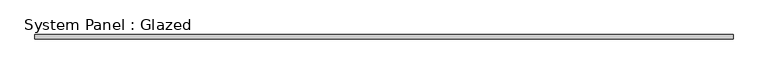
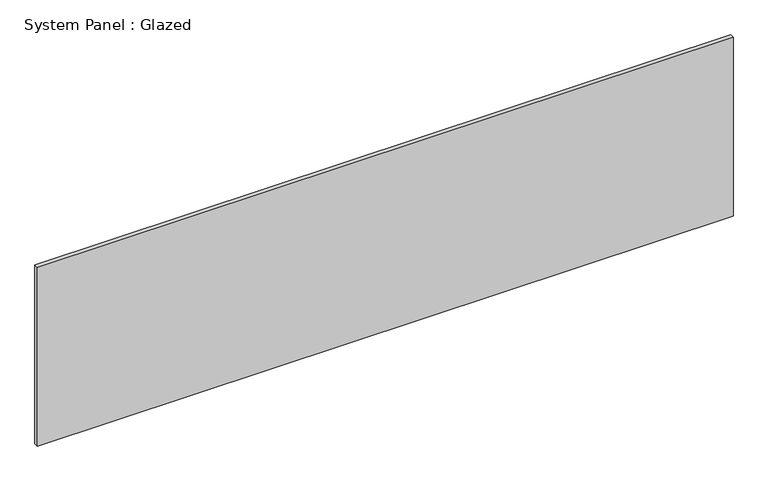
"""IFC4 building model written with IfcOpenShell, lengths in millimetres: plate geometry, System Panel : Glazed."""

from ifc_helpers import new_model, si_unit, origin, origin_with_axes, place, context, project, spatial, polyline, outline, extrude, source, transform, mapped, element, save


def system_panel_glazed_93b9a344(model_context):
    return source(origin(), model_context, "Body", "SweptSolid", [
        extrude(outline(polyline([(2009.775, 19.05), (-2009.775, 19.05), (-2009.775, 44.45), (2009.775, 44.45), (2009.775, 19.05)])), origin_with_axes(), (0.0, 0.0, 1.0), 1092.2),
    ])


if __name__ == "__main__":
    model = new_model("IFC4")
    model_context = context("Model", 3, world=origin())
    ifc_project = project(units=[si_unit("LENGTHUNIT", "METRE", prefix="MILLI")], contexts=[model_context])
    site = spatial("IfcSite", under=ifc_project)
    building = spatial("IfcBuilding", under=site)
    placement = place(None, origin())
    system_panel_glazed_shape = system_panel_glazed_93b9a344(model_context)
    element("IfcPlate", 1, ObjectType="System Panel : Glazed", at=placement, inside=building, context=model_context, shape_type="MappedRepresentation", body=[
        mapped(system_panel_glazed_shape, transform((0.0, 0.0, 0.0), x_axis=(1.0, 0.0, 0.0), y_axis=(0.0, 1.0, 0.0), z_axis=(0.0, 0.0, 1.0))),
    ])
    save(model, "model.ifc")

# Revit data of these elements
# Type "System Panel : Glazed"
#   Construction Type Id = "GSP4R"
#   Analytic Construction = "1/8 in Pilkington single glazing"
#   Visual Light Transmittance = 0.9
#   Solar Heat Gain Coefficient = 0.86
#   Heat Transfer Coefficient (U) = 1.18115 BTU/(h·ft²·°F)
# Element 1 (IfcPlate, "System Panel : Glazed")
#   Materials on its faces: "Glass"
# Materials
#   "Glass": class "Glass", colour RGB 0 128 192, transparency 0.75, Description = "Soda Lime Glass", Cost = 0
